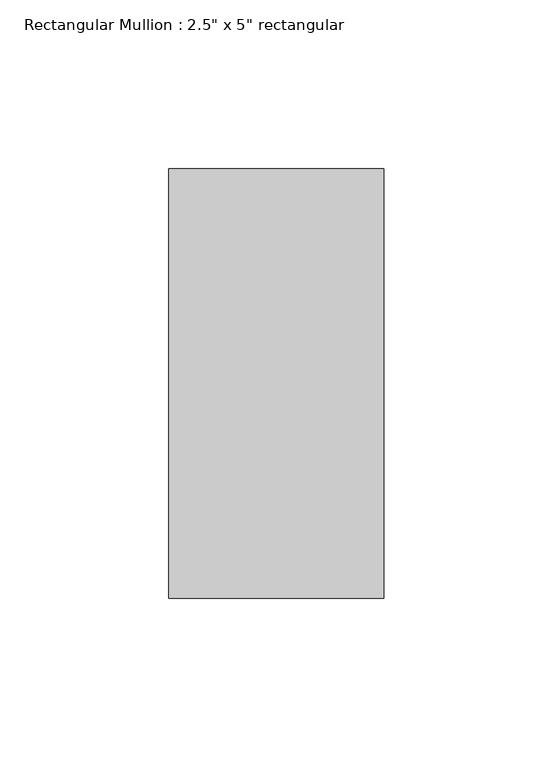
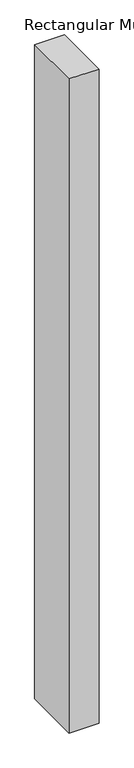
"""IFC4 building model written with IfcOpenShell, lengths in millimetres: member geometry."""

from ifc_helpers import new_model, si_unit, frame, origin, place, context, project, spatial, polyline, outline, extrude, source, transform, mapped, element, save


def member_53df7686(model_context):
    return source(origin(), model_context, "Body", "SweptSolid", [
        extrude(outline(polyline([(31.75, 63.5), (31.75, -63.5), (-31.75, -63.5), (-31.75, 63.5), (31.75, 63.5)])), frame((0.0, 0.0, -1472.6043316), z_axis=(0.0, 0.0, 1.0), x_axis=(1.0, 0.0, 0.0)), (0.0, 0.0, 1.0), 1472.6043316),
    ])


if __name__ == "__main__":
    model = new_model("IFC4")
    model_context = context("Model", 3, world=origin())
    ifc_project = project(units=[si_unit("LENGTHUNIT", "METRE", prefix="MILLI")], contexts=[model_context])
    site = spatial("IfcSite", under=ifc_project)
    building = spatial("IfcBuilding", under=site)
    placement = place(None, origin())
    member_shape = member_53df7686(model_context)
    element("IfcMember", 1, ObjectType="Rectangular Mullion : 2.5\" x 5\" rectangular", at=placement, inside=building, context=model_context, shape_type="MappedRepresentation", body=[
        mapped(member_shape, transform((0.0, 0.0, 0.0), x_axis=(1.0, 0.0, 0.0), y_axis=(0.0, 1.0, 0.0), z_axis=(0.0, 0.0, 1.0))),
    ])
    save(model, "model.ifc")

# Revit data of these elements
# Type "Rectangular Mullion : 2.5\" x 5\" rectangular"
#   built-in parameter 1007304 = 0.416667 (stored number, unit not read)
#   built-in parameter 1007301 = 0.104167 (stored number, unit not read)
#   built-in parameter 1007300 = 0.104167 (stored number, unit not read)
# Element 1 (IfcMember, "Rectangular Mullion : 2.5\" x 5\" rectangular")
#   Materials on its faces: "Aluminum"
# Materials
#   "Aluminum": class "Metal", colour RGB 247 247 247, transparency 0, Description = "Aluminum 6061", Cost = 0
